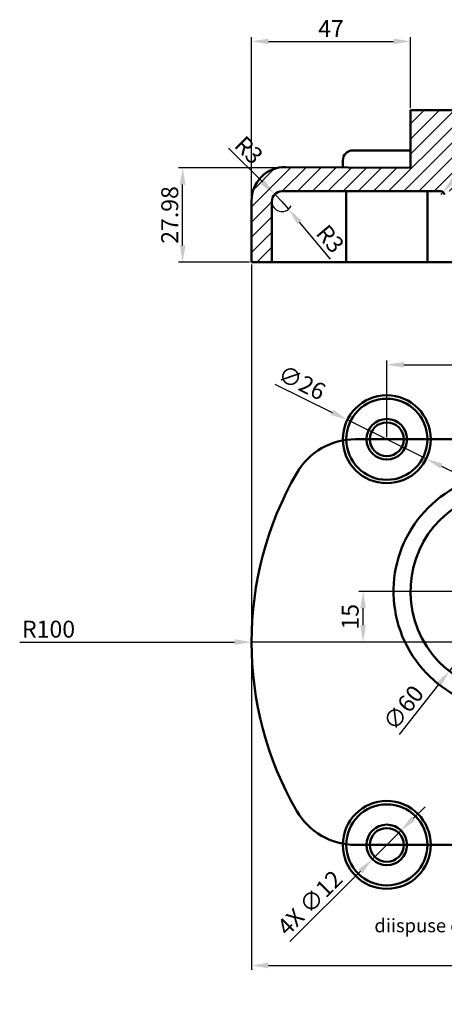
# Model space of a CAD drawing. Units: millimetres. Extents: x 2983 to 3450, y 1738 to 2029.
# Tile 1 of 3: x 2983 to 3108, y 1738 to 2029. Entities that reach past the tile are written whole.
import ezdxf
from ezdxf import colors
from ezdxf.entities.mleader import LeaderData, LeaderLine
from ezdxf.math import Vec2, Vec3

# ---------------------------------------------------------------- set-up
doc = ezdxf.new("R2010")
doc.units = ezdxf.units.MM
for name, color, linetype, lineweight in [('M-DIMS', 2, 'Continuous', 25), ('M-HATC', 8, 'Continuous', 18), ('M-OUTL', 7, 'Continuous', 50)]:
    doc.layers.add(name, color=color, linetype=linetype, lineweight=lineweight)
doc.styles.get("Standard").update_dxf_attribs({"font": 'arial.ttf'})
doc.dimstyles.new('ISO-25', dxfattribs={"dimtxt": 5, "dimasz": 5, "dimexe": 1.25, "dimexo": 0.625, "dimtad": 1, "dimdec": 0, "dimtxsty": 'Standard', "dimcen": 2.5, "dimadec": 0, "dimazin": 0, "dimtfac": 1, "dimtdec": 0, "dimtmove": 0, "dimatfit": 3, "dimfxl": 1, "dimarcsym": 0})

# ---------------------------------------------------------------- blocks, each defined once
blk = doc.blocks.new('*D4')
at = {"layer": 'Defpoints', "color": 0, "transparency": 16777216}
for p in [(3205.47, 1927.36), (3091.47, 1905.31), (3205.47, 1905.31)]:
    blk.add_point(p, dxfattribs=at)
at = {"layer": 'M-DIMS', "color": 0, "lineweight": -2, "transparency": 16777216}
for p, q in [((3091.47, 1905.94), (3091.47, 1928.61)), ((3205.47, 1905.94), (3205.47, 1928.61)), ((3096.47, 1927.36), (3200.47, 1927.36))]:
    blk.add_line(p, q, dxfattribs=at)
at = {"layer": 'M-DIMS', "color": 0, "transparency": 16777216}
for points in [[(3096.47, 1928.19), (3096.47, 1926.52), (3091.47, 1927.36)], [(3200.47, 1928.19), (3200.47, 1926.52), (3205.47, 1927.36)]]:
    blk.add_solid(points, dxfattribs=at)
at = {"layer": 'M-DIMS', "color": 0, "transparency": 16777216, "insert": (3148.47, 1930.49), "char_height": 5, "attachment_point": 5}
blk.add_mtext('114', dxfattribs=at)
blk = doc.blocks.new('*D10')
at = {"layer": 'Defpoints', "color": 0, "transparency": 16777216}
for p in [(3084.47, 1860.31), (3128.47, 1860.31), (3188.47, 1845.31)]:
    blk.add_point(p, dxfattribs=at)
at = {"layer": 'M-DIMS', "color": 0, "lineweight": -2, "transparency": 16777216}
for p, q in [((3127.85, 1860.31), (3083.22, 1860.31)), ((3084.47, 1850.31), (3084.47, 1855.31)), ((3187.85, 1845.31), (3083.22, 1845.31))]:
    blk.add_line(p, q, dxfattribs=at)
at = {"layer": 'M-DIMS', "color": 0, "transparency": 16777216}
for points in [[(3083.64, 1855.31), (3085.3, 1855.31), (3084.47, 1860.31)], [(3083.64, 1850.31), (3085.3, 1850.31), (3084.47, 1845.31)]]:
    blk.add_solid(points, dxfattribs=at)
at = {"layer": 'M-DIMS', "color": 0, "transparency": 16777216, "insert": (3081.29, 1852.81), "char_height": 5, "attachment_point": 5, "rotation": 90}
blk.add_mtext('15', dxfattribs=at)
blk = doc.blocks.new('*D11')
at = {"layer": 'Defpoints', "color": 0, "transparency": 16777216}
for p in [(3079.81, 1911.05), (3103.14, 1899.57)]:
    blk.add_point(p, dxfattribs=at)
at = {"layer": 'M-DIMS', "color": 0, "lineweight": -2, "transparency": 16777216}
for p, q in [((3058.41, 1921.58), (3075.32, 1913.26)), ((3103.14, 1899.57), (3079.81, 1911.05)), ((3107.63, 1897.37), (3112.11, 1895.16))]:
    blk.add_line(p, q, dxfattribs=at)
at = {"layer": 'M-DIMS', "color": 0, "transparency": 16777216}
for points in [[(3075.69, 1914.01), (3074.96, 1912.51), (3079.81, 1911.05)], [(3107.99, 1898.11), (3107.26, 1896.62), (3103.14, 1899.57)]]:
    blk.add_solid(points, dxfattribs=at)
at = {"layer": 'M-DIMS', "color": 0, "transparency": 16777216, "insert": (3066.09, 1921.5), "char_height": 5, "attachment_point": 5, "rotation": 333.8021}
blk.add_mtext('∅26', dxfattribs=at)
blk = doc.blocks.new('*D14')
at = {"layer": 'Defpoints', "color": 0, "transparency": 16777216}
for p in [(3147.01, 1883.9), (3109.94, 1836.72)]:
    blk.add_point(p, dxfattribs=at)
at = {"layer": 'M-DIMS', "color": 0, "lineweight": -2, "transparency": 16777216}
for p, q in [((3150.09, 1887.84), (3153.18, 1891.77)), ((3147.01, 1883.9), (3109.94, 1836.72)), ((3095.22, 1817.98), (3106.85, 1832.79))]:
    blk.add_line(p, q, dxfattribs=at)
at = {"layer": 'M-DIMS', "color": 0, "transparency": 16777216}
for points in [[(3149.44, 1888.35), (3150.75, 1887.32), (3147.01, 1883.9)], [(3106.2, 1833.3), (3107.51, 1832.27), (3109.94, 1836.72)]]:
    blk.add_solid(points, dxfattribs=at)
at = {"layer": 'M-DIMS', "color": 0, "transparency": 16777216, "insert": (3096.88, 1825.47), "char_height": 5, "attachment_point": 5, "rotation": 51.8501}
blk.add_mtext('∅60', dxfattribs=at)
blk = doc.blocks.new('*D25')
at = {"layer": 'Defpoints', "color": 0, "transparency": 16777216}
for p in [(3060.47, 1975.67), (3062.41, 1973.38)]:
    blk.add_point(p, dxfattribs=at)
at = {"layer": 'M-DIMS', "color": 0, "lineweight": -2, "transparency": 16777216}
for p, q in [((3060.47, 1975.67), (3062.41, 1973.38)), ((3074.84, 1958.59), (3065.62, 1969.55))]:
    blk.add_line(p, q, dxfattribs=at)
blk.add_arc((3060.47, 1975.67), 3, 191.9366, 333.9355, dxfattribs=at)
at = {"layer": 'M-DIMS', "color": 0, "transparency": 16777216}
blk.add_solid([(3066.26, 1970.08), (3064.99, 1969.01), (3062.41, 1973.38)], dxfattribs=at)
at = {"layer": 'M-DIMS', "color": 0, "transparency": 16777216, "insert": (3074.27, 1964.2), "char_height": 5, "attachment_point": 5, "rotation": 310.0623}
blk.add_mtext('R3', dxfattribs=at)
blk = doc.blocks.new('CBORE-HOLE')
for radius in [13, 12, 6, 5]:
    blk.add_circle((3205.47, 1905.31), radius)
blk = doc.blocks.new('*D36')
at = {"layer": 'Defpoints', "color": 0, "transparency": 16777216}
for p in [(3051.47, 1957.67), (3248.47, 1957.67), (3248.47, 1749.65)]:
    blk.add_point(p, dxfattribs=at)
at = {"layer": 'M-DIMS', "color": 0, "lineweight": -2, "transparency": 16777216}
for p, q in [((3051.47, 1957.05), (3051.47, 1748.4)), ((3248.47, 1957.05), (3248.47, 1748.4)), ((3056.47, 1749.65), (3243.47, 1749.65))]:
    blk.add_line(p, q, dxfattribs=at)
at = {"layer": 'M-DIMS', "color": 0, "transparency": 16777216}
for points in [[(3056.47, 1750.48), (3056.47, 1748.81), (3051.47, 1749.65)], [(3243.47, 1750.48), (3243.47, 1748.81), (3248.47, 1749.65)]]:
    blk.add_solid(points, dxfattribs=at)
at = {"layer": 'M-DIMS', "color": 0, "transparency": 16777216, "insert": (3149.97, 1752.82), "char_height": 5, "attachment_point": 5}
blk.add_mtext('197', dxfattribs=at)
blk = doc.blocks.new('*D37')
at = {"layer": 'Defpoints', "color": 0, "transparency": 16777216}
for p in [(3098.47, 2023.02), (3098.47, 2002.67), (3051.47, 1957.67)]:
    blk.add_point(p, dxfattribs=at)
at = {"layer": 'M-DIMS', "color": 0, "lineweight": -2, "transparency": 16777216}
for p, q in [((3051.47, 1958.3), (3051.47, 2024.27)), ((3056.47, 2023.02), (3093.47, 2023.02)), ((3098.47, 2003.3), (3098.47, 2024.27))]:
    blk.add_line(p, q, dxfattribs=at)
at = {"layer": 'M-DIMS', "color": 0, "transparency": 16777216}
for points in [[(3056.47, 2023.85), (3056.47, 2022.19), (3051.47, 2023.02)], [(3093.47, 2023.85), (3093.47, 2022.19), (3098.47, 2023.02)]]:
    blk.add_solid(points, dxfattribs=at)
at = {"layer": 'M-DIMS', "color": 0, "transparency": 16777216, "insert": (3074.97, 2026.15), "char_height": 5, "attachment_point": 5}
blk.add_mtext('47', dxfattribs=at)
blk = doc.blocks.new('*D38')
at = {"layer": 'Defpoints', "color": 0, "transparency": 16777216}
for p in [(3031.12, 1985.65), (3098.47, 1985.65), (3051.47, 1957.67)]:
    blk.add_point(p, dxfattribs=at)
at = {"layer": 'M-DIMS', "color": 0, "lineweight": -2, "transparency": 16777216}
for p, q in [((3097.85, 1985.65), (3029.87, 1985.65)), ((3031.12, 1962.67), (3031.12, 1980.65)), ((3050.85, 1957.67), (3029.87, 1957.67))]:
    blk.add_line(p, q, dxfattribs=at)
at = {"layer": 'M-DIMS', "color": 0, "transparency": 16777216}
for points in [[(3030.29, 1980.65), (3031.96, 1980.65), (3031.12, 1985.65)], [(3030.29, 1962.67), (3031.96, 1962.67), (3031.12, 1957.67)]]:
    blk.add_solid(points, dxfattribs=at)
at = {"layer": 'M-DIMS', "color": 0, "transparency": 16777216, "insert": (3027.95, 1971.66), "char_height": 5, "attachment_point": 5, "rotation": 90}
blk.add_mtext('27.98', dxfattribs=at)
blk = doc.blocks.new('*D40')
at = {"layer": 'Defpoints', "color": 0, "transparency": 16777216}
for p in [(3095.72, 1789.55), (3087.23, 1781.07)]:
    blk.add_point(p, dxfattribs=at)
at = {"layer": 'M-DIMS', "color": 0, "lineweight": -2, "transparency": 16777216}
for p, q in [((3099.26, 1793.09), (3102.79, 1796.62)), ((3095.72, 1789.55), (3087.23, 1781.07)), ((3062.84, 1756.7), (3083.69, 1777.54))]:
    blk.add_line(p, q, dxfattribs=at)
at = {"layer": 'M-DIMS', "color": 0, "transparency": 16777216}
for points in [[(3098.67, 1793.68), (3099.84, 1792.5), (3095.72, 1789.55)], [(3083.1, 1778.13), (3084.28, 1776.95), (3087.23, 1781.07)]]:
    blk.add_solid(points, dxfattribs=at)
at = {"layer": 'M-DIMS', "color": 0, "transparency": 16777216, "insert": (3069.15, 1767.7), "char_height": 5, "attachment_point": 5, "rotation": 44.9791}
blk.add_mtext('4X ∅12', dxfattribs=at)
blk = doc.blocks.new('*D42')
at = {"layer": 'Defpoints', "color": 0, "transparency": 16777216}
for p in [(3051.47, 1845.31), (3151.47, 1845.31)]:
    blk.add_point(p, dxfattribs=at)
at = {"layer": 'M-DIMS', "color": 0, "lineweight": -2, "transparency": 16777216}
for p, q in [((2982.94, 1845.31), (3046.47, 1845.31)), ((3151.47, 1845.31), (3051.47, 1845.31))]:
    blk.add_line(p, q, dxfattribs=at)
at = {"layer": 'M-DIMS', "color": 0, "transparency": 16777216}
blk.add_solid([(3046.47, 1846.15), (3046.47, 1844.48), (3051.47, 1845.31)], dxfattribs=at)
at = {"layer": 'M-DIMS', "color": 0, "transparency": 16777216, "insert": (2991.47, 1848.49), "char_height": 5, "attachment_point": 5, "rotation": 359.9998}
blk.add_mtext('R100', dxfattribs=at)
blk = doc.blocks.new('*D45')
at = {"layer": 'Defpoints', "color": 0, "transparency": 16777216}
for p in [(3058.35, 1977.79), (3060.47, 1975.67)]:
    blk.add_point(p, dxfattribs=at)
at = {"layer": 'M-DIMS', "color": 0, "lineweight": -2, "transparency": 16777216}
for p, q in [((3044.7, 1991.45), (3054.82, 1981.33)), ((3060.47, 1975.67), (3058.35, 1977.79))]:
    blk.add_line(p, q, dxfattribs=at)
at = {"layer": 'M-DIMS', "color": 0, "transparency": 16777216}
blk.add_solid([(3055.41, 1981.92), (3054.23, 1980.74), (3058.35, 1977.79)], dxfattribs=at)
at = {"layer": 'M-DIMS', "color": 0, "transparency": 16777216, "insert": (3050.24, 1990.4), "char_height": 5, "attachment_point": 5, "rotation": 315}
blk.add_mtext('R3', dxfattribs=at)
blk = doc.blocks.new('*D46')
at = {"layer": 'Defpoints', "color": 0, "transparency": 16777216}
for p in [(3108.14, 1978.42), (3107.47, 1977.67)]:
    blk.add_point(p, dxfattribs=at)
at = {"layer": 'M-DIMS', "color": 0, "lineweight": -2, "transparency": 16777216}
for p, q in [((3120.33, 1992.13), (3111.46, 1982.16)), ((3107.47, 1977.67), (3108.14, 1978.42))]:
    blk.add_line(p, q, dxfattribs=at)
at = {"layer": 'M-DIMS', "color": 0, "transparency": 16777216}
blk.add_solid([(3110.84, 1982.71), (3112.08, 1981.6), (3108.14, 1978.42)], dxfattribs=at)
at = {"layer": 'M-DIMS', "color": 0, "transparency": 16777216, "insert": (3115.21, 1991.1), "char_height": 5, "attachment_point": 5, "rotation": 48.3754}
blk.add_mtext('R1', dxfattribs=at)

msp = doc.modelspace()

# ---------------------------------------------------------------- hatches: boundary and pattern name
at = {"layer": 'M-HATC'}
h = msp.add_hatch(dxfattribs=at)
h.set_pattern_fill('ANSI31', color=256)
h.set_pattern_definition([(45, (0, -22.2306), (-2.245064, 2.245064), [])])
h.paths.add_polyline_path([(3114.475, 1997.671), (3110.975, 1997.671), (3110.975, 2002.671), (3098.475, 2002.671), (3098.475, 1985.65), (3061.528, 1985.846, 0.4157622), (3051.475, 1975.846), (3051.475, 1957.671), (3057.475, 1957.671), (3057.475, 1975.671, -0.4142136), (3060.475, 1978.671), (3079.476, 1978.671), (3103.475, 1978.671), (3110.475, 1978.671, -0.4142136), (3111.475, 1977.671), (3111.475, 1976.671), (3114.475, 1976.671)])
h.paths.add_polyline_path([(3164.888, 2001.611), (3163.828, 2002.671), (3145.975, 2002.671), (3145.975, 1997.671), (3142.475, 1997.671), (3142.475, 1976.671), (3146.337, 1976.671, -0.4142136), (3148.337, 1978.671), (3159.52, 1978.671, -0.4142136), (3161.52, 1976.671), (3164.888, 1976.671), (3164.888, 1978.671)])
h.paths.add_polyline_path([(3216.888, 1978.671), (3240.475, 1978.671, -0.4142136), (3242.475, 1976.671), (3242.475, 1957.671), (3248.475, 1957.671), (3248.475, 1972.671, 0.4142136), (3238.475, 1982.671), (3232.475, 1982.671, -0.4142136), (3229.475, 1985.671), (3229.475, 2002.671), (3209.535, 2002.671), (3208.475, 2001.611), (3208.475, 1976.671), (3214.888, 1976.671, -0.4142136)])

# ---------------------------------------------------------------- linework, layer by layer
at = {"layer": 'M-OUTL'}
for p, q in [((3110.975, 2002.671), (3098.475, 2002.671)), ((3098.475, 2002.671), (3098.475, 1985.65)), ((3081.475, 1990.756), (3098.475, 1990.756)), ((3078.475, 1985.756), (3078.475, 1987.756)), ((3098.475, 1985.65), (3061.528, 1985.846)), ((3079.476, 1978.671), (3060.475, 1978.671)), ((3079.476, 1978.671), (3107.475, 1978.671)), ((3079.476, 1957.671), (3079.476, 1978.671)), ((3103.475, 1957.671), (3103.475, 1978.671)), ((3051.475, 1975.846), (3051.475, 1957.671)), ((3057.475, 1957.671), (3057.475, 1975.671)), ((3051.475, 1957.671), (3248.475, 1957.671)), ((3051.475, 1957.671), (3057.475, 1957.671)), ((3091.475, 1905.312), (3082.193, 1905.312)), ((3205.475, 1905.312), (3091.475, 1905.312)), ((3091.475, 1785.312), (3082.193, 1785.312)), ((3091.475, 1785.312), (3205.475, 1785.312))]:
    msp.add_line(p, q, dxfattribs=at)
for centre, radius, start, end in [((3081.475, 1987.756), 3, 90, 180), ((3061.475, 1975.846), 10, 89.69722, 180), ((3060.475, 1975.671), 3, 90, 180), ((3107.475, 1977.671), 1, 0, 90), ((3082.193, 1885.312), 20, 90, 150), ((3151.475, 1845.312), 100, 150, 210), ((3128.475, 1860.312), 35, 41.16002, 290.7675), ((3128.475, 1860.312), 30, 41.16002, 290.7675), ((3082.193, 1805.312), 20, 210, 270)]:
    msp.add_arc(centre, radius, start, end, dxfattribs=at)

# ---------------------------------------------------------------- block references
for p in [(-114, 0), (-114, -120)]:
    msp.add_blockref('CBORE-HOLE', p, dxfattribs=at)

# ---------------------------------------------------------------- dimensions: what is measured, and where the dimension line sits
at = {"layer": 'M-DIMS'}
for base, p1, p2, override, picture, middle in [((3098.475, 2023.021), (3051.475, 1957.671), (3098.475, 2002.671), {"dimdec": 0, "dimlfac": 1, "dimrnd": 0, "dimzin": 0, "dimdsep": 46, "dimlunit": 2}, '*D37', (3074.975, 2026.146)), ((3248.475, 1749.646), (3051.475, 1957.671), (3248.475, 1957.671), {"dimdec": 0, "dimlfac": 1, "dimrnd": 0, "dimzin": 0, "dimdsep": 46, "dimlunit": 2}, '*D36', (3149.975, 1752.824)), ((3205.475, 1927.357), (3091.475, 1905.312), (3205.475, 1905.312), {"dimclrd": 0, "dimclre": 0, "dimclrt": 0}, '*D4', (3148.475, 1930.492))]:
    dim = msp.add_linear_dim(base=base, p1=p1, p2=p2, dimstyle='ISO-25', override=override, dxfattribs=at)
    dim.commit()
    dim.dimension.update_dxf_attribs({"geometry": picture, "text_midpoint": middle})
for center, mpoint, override, picture, middle in [((3060.475, 1975.671), (3058.353, 1977.793), {"dimdec": 0, "dimlfac": 1, "dimrnd": 0, "dimzin": 0, "dimdsep": 46, "dimlunit": 2}, '*D45', (3050.238, 1990.404)), ((3107.475, 1977.671), (3108.139, 1978.419), {"dimdec": 0, "dimlfac": 1, "dimrnd": 0, "dimzin": 0, "dimdsep": 46, "dimlunit": 2}, '*D46', (3115.21, 1991.096)), ((3060.475, 1975.671), (3062.406, 1973.375), {"dimclrd": 0, "dimclre": 0, "dimclrt": 0}, '*D25', (3074.272, 1964.204))]:
    dim = msp.add_radius_dim(center=center, mpoint=mpoint, dimstyle='ISO-25', override=override, dxfattribs=at)
    dim.commit()
    dim.dimension.update_dxf_attribs({"geometry": picture, "text_midpoint": middle})
for base, p1, p2, override, picture, middle in [((3031.125, 1985.65), (3051.475, 1957.671), (3098.475, 1985.65), {"dimdec": 2, "dimlfac": 1, "dimrnd": 0, "dimzin": 0, "dimdsep": 46, "dimlunit": 2}, '*D38', (3027.947, 1971.661)), ((3084.469, 1860.312), (3188.475, 1845.312), (3128.475, 1860.312), {"dimclrd": 0, "dimclre": 0, "dimclrt": 0}, '*D10', (3081.291, 1852.812))]:
    dim = msp.add_linear_dim(base=base, p1=p1, p2=p2, angle=90, dimstyle='ISO-25', override=override, dxfattribs=at)
    dim.commit()
    dim.dimension.update_dxf_attribs({"geometry": picture, "text_midpoint": middle})
for p1, p2, picture, middle in [((3103.139, 1899.572), (3079.81, 1911.051), '*D11', (3064.624, 1918.522)), ((3147.006, 1883.904), (3109.943, 1836.72), '*D14', (3096.884, 1825.465))]:
    dim = msp.add_diameter_dim_2p(p1=p1, p2=p2, dimstyle='ISO-25', override={"dimclrd": 0, "dimclre": 0, "dimclrt": 0}, dxfattribs=at)
    dim.commit()
    dim.dimension.update_dxf_attribs({"geometry": picture, "text_midpoint": middle})
dim = msp.add_radius_dim(center=(3151.475, 1845.312), mpoint=(3051.475, 1845.312), dimstyle='ISO-25', override={"dimdec": 0, "dimlfac": 1, "dimrnd": 0, "dimzin": 0, "dimdsep": 46, "dimlunit": 2}, dxfattribs=at)
dim.commit()
dim.dimension.update_dxf_attribs({"geometry": '*D42', "text_midpoint": (2991.475, 1845.312), "dimtype": 164})
dim = msp.add_diameter_dim_2p(p1=(3095.719, 1789.553), p2=(3087.231, 1781.071), text='4X <>', dimstyle='ISO-25', override={"dimdec": 0, "dimlfac": 1, "dimrnd": 0, "dimzin": 0, "dimdsep": 46, "dimlunit": 2}, dxfattribs=at)
dim.commit()
dim.dimension.update_dxf_attribs({"geometry": '*D40', "text_midpoint": (3071.499, 1765.35), "dimtype": 163})

# ---------------------------------------------------------------- leaders
ml = msp.add_multileader_mtext('Standard', dxfattribs=at)
ml.set_content('6 gauri M12\\Pdiispuse echididtant', color=256)
ml.set_leader_properties()
ml.build(insert=Vec2(0, 0))
ctx = ml.context
ctx.base_point, ctx.plane_origin = Vec3(3088.784, 1767.575), Vec3(3161.337, 1824.105)
ctx.text_align_type = 2
notes = []
notes.append((ctx, [(0, (1, 1, 0), (3149.635, 1767.575), (-1, 0), 8, [(0, [(3161.337, 1824.105)], 0, [])])]))
ctx.mtext.insert, ctx.mtext.alignment, ctx.mtext.flow_direction = Vec3(3139.635, 1770.13), 3, 5
for ctx, leaders in notes:
    for number, flags, end, landing, length, lines in leaders:
        leader = LeaderData()
        leader.index, (leader.has_last_leader_line, leader.has_dogleg_vector, leader.attachment_direction) = number, flags
        leader.last_leader_point, leader.dogleg_vector, leader.dogleg_length = Vec3(end), Vec3(landing), length
        for number, points, colour, breaks in lines:
            line = LeaderLine()
            line.index, line.vertices, line.color, line.breaks = number, Vec3.list(points), colors.encode_raw_color(colour), breaks
            leader.lines.append(line)
        ctx.leaders.append(leader)

doc.saveas('drawing.dxf')
